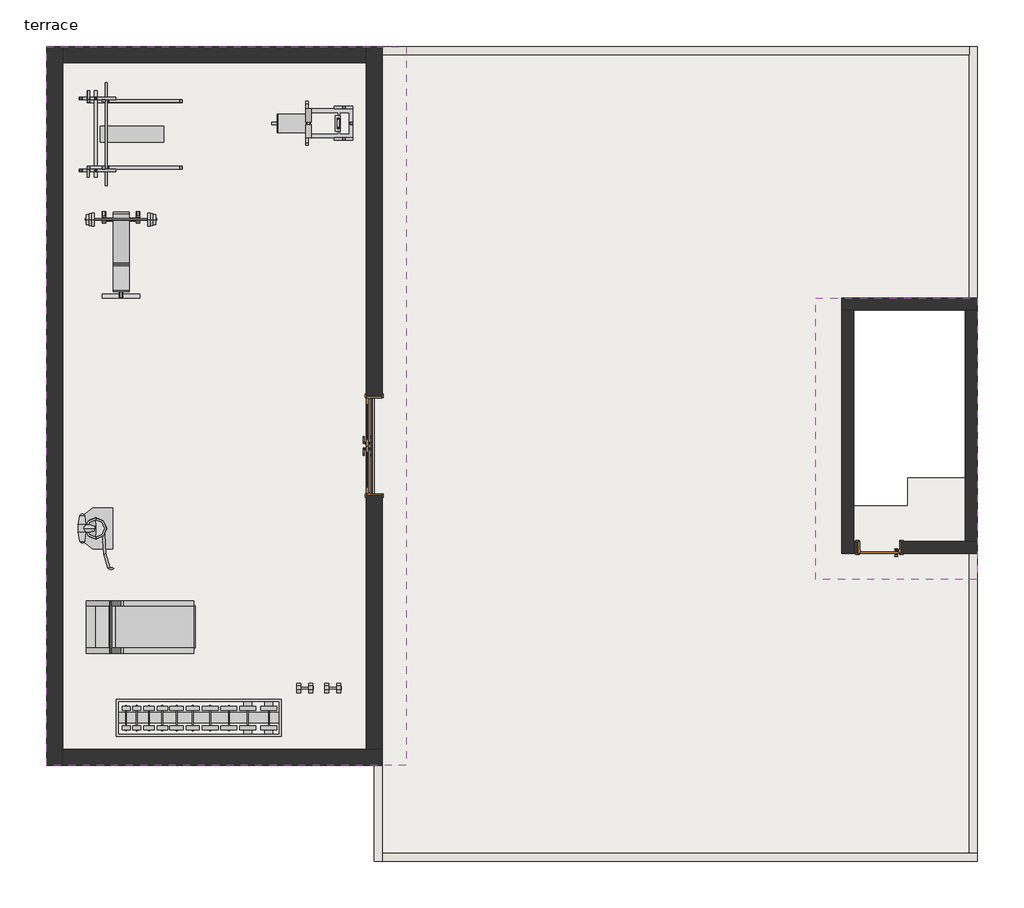
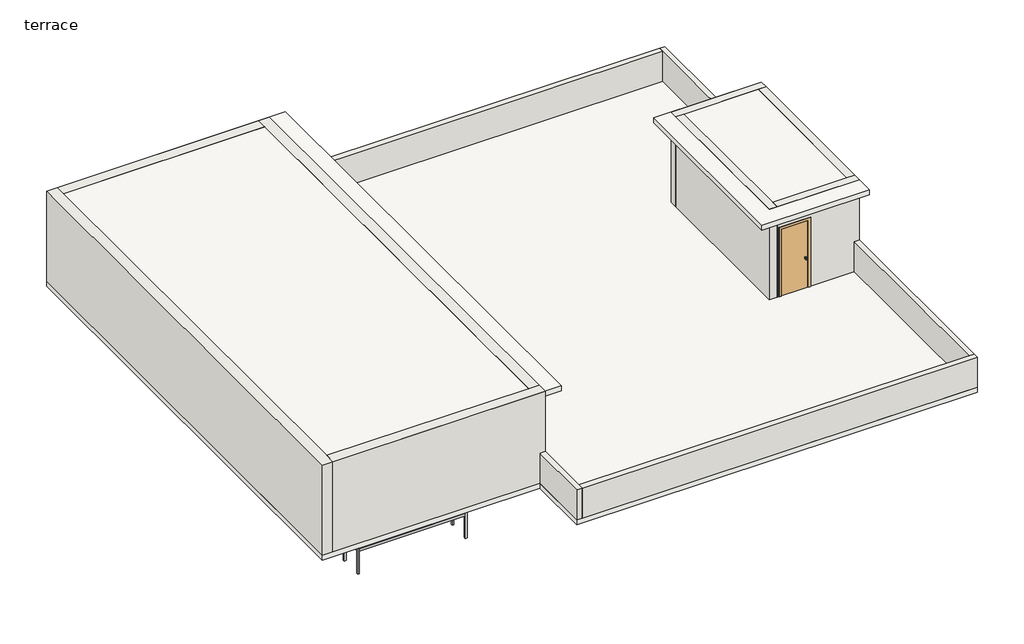
# One storey, incomplete: 13 walls, 7 proxies, 3 slabs, 2 doors, 1 furniture element.
"""IFC4 building model written with IfcOpenShell, lengths in millimetres."""

from ifc_helpers import new_model, si_unit, frame, origin, place, context, project, spatial, polyline, outline, extrude, faceted_brep, transform, mapped, element, save
from components import generic_models_aa191242, specialty_equipment_60971a7b, generic_models_59bf1475, specialty_equipment_45cd0696, lifting_bench_lifting_bench_243d69f3, treadmill_metric_18420_treadmill_metric_18420_532483b1, door_c1904fbe, door_d1f25229, gym_weight_bench_set_14865_gym_weight_bench_set_14865_0f5544b4

model = new_model("IFC4")

# Units and contexts
model_context = context("Model", 3, world=origin())
ifc_project = project(units=[si_unit("LENGTHUNIT", "METRE", prefix="MILLI")], contexts=[model_context])

# Site, building, storey
site = spatial("IfcSite", under=ifc_project)
building = spatial("IfcBuilding", under=site)
storey = spatial("IfcBuildingStorey", under=building, Name="terrace", Elevation=10210.8)

# Proxies
placement = place(None, origin())
generic_models_shape = generic_models_aa191242(model_context)
element("IfcBuildingElementProxy", 1, Name="Generic Models", at=placement, inside=storey, context=model_context, shape_type="MappedRepresentation", body=[
    mapped(generic_models_shape, transform((-7089.7739162, -2120.8339187, 10210.8), x_axis=(0.0, 1.0, 0.0), y_axis=(-1.0, 0.0, 0.0), z_axis=(0.0, 0.0, 1.0))),
])
specialty_equipment_shape = specialty_equipment_60971a7b(model_context)
element("IfcBuildingElementProxy", 2, Name="Specialty Equipment", at=placement, inside=storey, context=model_context, shape_type="MappedRepresentation", body=[
    mapped(specialty_equipment_shape, transform((-5667.3739162, -5930.8339187, 10210.8), x_axis=(1.0, 0.0, 0.0), y_axis=(0.0, 1.0, 0.0), z_axis=(0.0, 0.0, 1.0))),
])
generic_models_2_shape = generic_models_59bf1475(model_context)
element("IfcBuildingElementProxy", 3, Name="Generic Models", at=placement, inside=storey, context=model_context, shape_type="MappedRepresentation", body=[
    mapped(generic_models_2_shape, transform((-2644.7739162, -5168.8339187, 10210.8), x_axis=(1.0, 0.0, 0.0), y_axis=(0.0, 1.0, 0.0), z_axis=(0.0, 0.0, 1.0))),
])
element("IfcBuildingElementProxy", 4, Name="Generic Models", at=placement, inside=storey, context=model_context, shape_type="MappedRepresentation", body=[
    mapped(generic_models_2_shape, transform((-3178.1739162, -5168.8339187, 10210.8), x_axis=(1.0, 0.0, 0.0), y_axis=(0.0, 1.0, 0.0), z_axis=(0.0, 0.0, 1.0))),
])
specialty_equipment_2_shape = specialty_equipment_45cd0696(model_context)
element("IfcBuildingElementProxy", 5, Name="Specialty Equipment", at=placement, inside=storey, context=model_context, shape_type="MappedRepresentation", body=[
    mapped(specialty_equipment_2_shape, transform((-2429.0078371, 5204.0745668, 10210.8), x_axis=(0.0, 1.0, 0.0), y_axis=(-1.0, 0.0, 0.0), z_axis=(0.0, 0.0, 1.0))),
])
lifting_bench_lifting_bench_shape = lifting_bench_lifting_bench_243d69f3(model_context)
element("IfcBuildingElementProxy", 6, Name="Lifting Bench : Lifting Bench", ObjectType="Lifting Bench : Lifting Bench", at=placement, inside=storey, context=model_context, shape_type="MappedRepresentation", body=[
    mapped(lifting_bench_lifting_bench_shape, transform((-6964.4872648, 2273.3660813, 10210.8), x_axis=(1.0, 0.0, 0.0), y_axis=(0.0, 1.0, 0.0), z_axis=(0.0, 0.0, 1.0))),
])
treadmill_metric_18420_treadmill_metric_18420_shape = treadmill_metric_18420_treadmill_metric_18420_532483b1(model_context)
element("IfcBuildingElementProxy", 7, Name="Treadmill_metric_18420 : Treadmill_metric_18420", ObjectType="Treadmill_metric_18420 : Treadmill_metric_18420", at=placement, inside=storey, context=model_context, shape_type="MappedRepresentation", body=[
    mapped(treadmill_metric_18420_treadmill_metric_18420_shape, transform((-7267.5739162, -3640.5277171, 10210.8), x_axis=(0.0, -1.0, 0.0), y_axis=(1.0, 0.0, 0.0), z_axis=(0.0, 0.0, 1.0))),
])

# Doors
door_shape = door_c1904fbe(model_context)
element("IfcDoor", 8, ObjectType="Door-Exterior-Double-Full Glass-Wood_Clad : 72\" x 84\"", at=placement, inside=storey, context=model_context, shape_type="MappedRepresentation", body=[
    mapped(door_shape, transform((-1784.3489162, -546.0339187, 10210.8), x_axis=(0.0, 1.0, 0.0), y_axis=(-1.0, 0.0, 0.0), z_axis=(0.0, 0.0, 1.0))),
])
door_2_shape = door_d1f25229(model_context)
element("IfcDoor", 9, ObjectType="Door-Interior-Single-Flush_Panel-Wood : 30\" x 80\"", at=placement, inside=storey, context=model_context, shape_type="MappedRepresentation", body=[
    mapped(door_2_shape, transform((7858.1260838, -2492.3089187, 10210.8), x_axis=(-1.0, 0.0, 0.0), y_axis=(0.0, -1.0, 0.0), z_axis=(0.0, 0.0, 1.0))),
])

# Furniture
gym_weight_bench_set_14865_gym_weight_bench_set_14865_shape = gym_weight_bench_set_14865_gym_weight_bench_set_14865_0f5544b4(model_context)
element("IfcFurniture", 10, ObjectType="Gym_weight_bench_set_14865 : Gym_weight_bench_set_14865", at=placement, inside=storey, context=model_context, shape_type="MappedRepresentation", body=[
    mapped(gym_weight_bench_set_14865_gym_weight_bench_set_14865_shape, transform((-5438.7739162, 4737.1660813, 10210.8), x_axis=(0.0, 1.0, 0.0), y_axis=(-1.0, 0.0, 0.0), z_axis=(0.0, 0.0, 1.0))),
])

# Slabs
element("IfcSlab", 11, ObjectType="Generic - 6\"", at=placement, inside=storey, context=model_context, shape_type="SweptSolid", body=[
    extrude(outline(polyline([(-8029.5739162, 7073.9660813), (9725.0260838, 7073.9660813), (9725.0260838, 2044.7660813), (7362.8260838, 2044.7660813), (7362.8260838, -1689.0339187), (8391.5260838, -1689.0339187), (8391.5260838, -1157.2214187), (9725.0260838, -1157.2214187), (9725.0260838, -8470.8339187), (-1781.1739162, -8470.8339187), (-1781.1739162, -6642.0339187), (-8029.5739162, -6642.0339187), (-8029.5739162, 7073.9660813)])), frame((0.0, 0.0, 10058.4), z_axis=(0.0, 0.0, 1.0), x_axis=(1.0, 0.0, 0.0)), (0.0, 0.0, 1.0), 152.4),
])
element("IfcSlab", 12, ObjectType="Generic - 6\"", at=placement, inside=storey, context=model_context, shape_type="SweptSolid", body=[
    extrude(outline(polyline([(9725.0260838, 2273.3660813), (9725.0260838, -3098.7339187), (6638.9260838, -3098.7339187), (6638.9260838, 2273.3660813), (9725.0260838, 2273.3660813)])), frame((0.0, 0.0, 12801.6), z_axis=(0.0, 0.0, 1.0), x_axis=(1.0, 0.0, 0.0)), (0.0, 0.0, 1.0), 152.4),
])
element("IfcSlab", 13, ObjectType="Generic - 6\"", at=placement, inside=storey, context=model_context, shape_type="SweptSolid", body=[
    extrude(outline(polyline([(-1171.5739162, 7073.9660813), (-1171.5739162, -6642.0339187), (-8029.5739162, -6642.0339187), (-8029.5739162, 7073.9660813), (-1171.5739162, 7073.9660813)])), frame((0.0, 0.0, 12801.6), z_axis=(0.0, 0.0, 1.0), x_axis=(1.0, 0.0, 0.0)), (0.0, 0.0, 1.0), 152.4),
])

# Walls
element("IfcWall", 14, ObjectType="Generic - 12\"", at=placement, inside=storey, context=model_context, shape_type="Brep", body=[
    faceted_brep([(-8029.5739162, 7073.8999498, 10210.8), (-8029.5739162, -6642.0339187, 10210.8), (-8029.5739162, -6642.0339187, 12954.0), (-8029.5739162, 7073.8999498, 12954.0), (-7724.7739162, 7073.8999498, 10210.8), (-7724.7739162, 7073.8999498, 12954.0), (-7724.7739162, 6769.0999498, 12954.0), (-7724.7739162, -6337.2339187, 12954.0), (-7724.7739162, -6642.0339187, 12954.0), (-7724.7739162, -6642.0339187, 10210.8), (-7724.7739162, -6337.2339187, 10210.8), (-7724.7739162, 6769.0999498, 10210.8)], [[[0, 1, 2, 3]], [[4, 5, 6, 7, 8, 9, 10, 11]], [[1, 0, 4, 11, 10, 9]], [[3, 2, 8, 7, 6, 5]], [[2, 1, 9, 8]], [[0, 3, 5, 4]]]),
])
element("IfcWall", 15, ObjectType="Generic - 12\"", at=placement, inside=storey, context=model_context, shape_type="Brep", body=[
    faceted_brep([(-7724.7739162, -6642.0339187, 10210.8), (-1781.1739162, -6642.0339187, 10210.8), (-1781.1739162, -6642.0339187, 11125.2), (-1628.7739162, -6642.0339187, 11125.2), (-1628.7739162, -6642.0339187, 12954.0), (-7724.7739162, -6642.0339187, 12954.0), (-7724.7739162, -6337.2339187, 10210.8), (-7724.7739162, -6337.2339187, 12954.0), (-1933.5739162, -6337.2339187, 12954.0), (-1628.7739162, -6337.2339187, 12954.0), (-1628.7739162, -6337.2339187, 11125.2), (-1781.1739162, -6337.2339187, 11125.2), (-1781.1739162, -6337.2339187, 10210.8), (-1933.5739162, -6337.2339187, 10210.8)], [[[0, 1, 2, 3, 4, 5]], [[6, 7, 8, 9, 10, 11, 12, 13]], [[1, 0, 6, 13, 12]], [[5, 4, 9, 8, 7]], [[0, 5, 7, 6]], [[10, 3, 2, 11]], [[2, 1, 12, 11]], [[4, 3, 10, 9]]]),
])
element("IfcWall", 16, ObjectType="Generic - 12\"", at=placement, inside=storey, context=model_context, shape_type="SweptSolid", body=[
    extrude(outline(polyline([(-1933.5739162, 6769.0999498), (-7724.7739162, 6769.0999498), (-7724.7739162, 7073.8999498), (-1933.5739162, 7073.8999498), (-1933.5739162, 6769.0999498)])), frame((0.0, 0.0, 10210.8), z_axis=(0.0, 0.0, 1.0), x_axis=(1.0, 0.0, 0.0)), (0.0, 0.0, 1.0), 2743.2),
])
element("IfcWall", 17, ObjectType="Generic - 12\"", at=placement, inside=storey, context=model_context, shape_type="Brep", body=[
    faceted_brep([(-1933.5739162, -6337.2339187, 12954.0), (-1933.5739162, 6769.0999498, 12954.0), (-1933.5739162, 7073.9660813, 12954.0), (-1933.5739162, 7073.9660813, 10210.8), (-1933.5739162, 6769.0999498, 10210.8), (-1933.5739162, 393.7660813, 10210.8), (-1933.5739162, 393.7660813, 12369.8), (-1933.5739162, -1485.8339187, 12369.8), (-1933.5739162, -1485.8339187, 10210.8), (-1933.5739162, -6337.2339187, 10210.8), (-1628.7739162, 7073.9660813, 12954.0), (-1628.7739162, -6337.2339187, 12954.0), (-1628.7739162, -6337.2339187, 11125.2), (-1628.7739162, -6337.2339187, 10210.8), (-1628.7739162, -1485.8339187, 10210.8), (-1628.7739162, -1485.8339187, 12369.8), (-1628.7739162, 393.7660813, 12369.8), (-1628.7739162, 393.7660813, 10210.8), (-1628.7739162, 6921.5660813, 10210.8), (-1628.7739162, 7073.9660813, 10210.8), (-1628.7739162, 7073.9660813, 11125.2), (-1781.1739162, -6337.2339187, 10210.8)], [[[0, 1, 2, 3, 4, 5, 6, 7, 8, 9]], [[10, 11, 12, 13, 14, 15, 16, 17, 18, 19, 20]], [[3, 19, 18, 17, 5, 4]], [[13, 21, 9, 8, 14]], [[2, 1, 0, 11, 10]], [[3, 2, 10, 20, 19]], [[0, 9, 21, 13, 12, 11]], [[16, 6, 5, 17]], [[6, 16, 15, 7]], [[7, 15, 14, 8]]]),
])
element("IfcWall", 18, ObjectType="Generic - 6\"", at=placement, inside=storey, context=model_context, shape_type="Brep", body=[
    faceted_brep([(9725.0260838, 2273.3660813, 10210.8), (9725.0260838, 7073.9660813, 10210.8), (9725.0260838, 7073.9660813, 11125.2), (9725.0260838, 2273.3660813, 11125.2), (9572.6260838, 2273.3660813, 10210.8), (9572.6260838, 2273.3660813, 11125.2), (9572.6260838, 6921.5660813, 11125.2), (9572.6260838, 7073.9660813, 11125.2), (9572.6260838, 7073.9660813, 10210.8), (9572.6260838, 6921.5660813, 10210.8)], [[[0, 1, 2, 3]], [[4, 5, 6, 7, 8, 9]], [[1, 0, 4, 9, 8]], [[3, 2, 7, 6, 5]], [[0, 3, 5, 4]], [[2, 1, 8, 7]]]),
])
element("IfcWall", 19, ObjectType="Generic - 6\"", at=placement, inside=storey, context=model_context, shape_type="SweptSolid", body=[
    extrude(outline(polyline([(-1628.7739162, 7073.9660813), (9572.6260838, 7073.9660813), (9572.6260838, 6921.5660813), (-1628.7739162, 6921.5660813), (-1628.7739162, 7073.9660813)])), frame((0.0, 0.0, 10210.8), z_axis=(0.0, 0.0, 1.0), x_axis=(1.0, 0.0, 0.0)), (0.0, 0.0, 1.0), 914.4),
])
element("IfcWall", 20, ObjectType="Generic - 6\"", at=placement, inside=storey, context=model_context, shape_type="Brep", body=[
    faceted_brep([(-1781.1739162, -6337.2339187, 10210.8), (-1781.1739162, -6642.0339187, 10210.8), (-1781.1739162, -8470.8339187, 10210.8), (-1781.1739162, -8470.8339187, 11125.2), (-1781.1739162, -6642.0339187, 11125.2), (-1781.1739162, -6337.2339187, 11125.2), (-1628.7739162, -6337.2339187, 10210.8), (-1628.7739162, -6337.2339187, 11125.2), (-1628.7739162, -6642.0339187, 11125.2), (-1628.7739162, -8318.4339187, 11125.2), (-1628.7739162, -8470.8339187, 11125.2), (-1628.7739162, -8470.8339187, 10210.8), (-1628.7739162, -8318.4339187, 10210.8)], [[[0, 1, 2, 3, 4, 5]], [[6, 7, 8, 9, 10, 11, 12]], [[2, 1, 0, 6, 12, 11]], [[5, 4, 3, 10, 9, 8, 7]], [[3, 2, 11, 10]], [[0, 5, 7, 6]]]),
])
element("IfcWall", 21, ObjectType="Generic - 6\"", at=placement, inside=storey, context=model_context, shape_type="Brep", body=[
    faceted_brep([(-1628.7739162, -8470.8339187, 10210.8), (9725.0260838, -8470.8339187, 10210.8), (9725.0260838, -8470.8339187, 11125.2), (-1628.7739162, -8470.8339187, 11125.2), (-1628.7739162, -8318.4339187, 10210.8), (-1628.7739162, -8318.4339187, 11125.2), (9572.6260838, -8318.4339187, 11125.2), (9725.0260838, -8318.4339187, 11125.2), (9725.0260838, -8318.4339187, 10210.8), (9572.6260838, -8318.4339187, 10210.8)], [[[0, 1, 2, 3]], [[4, 5, 6, 7, 8, 9]], [[1, 0, 4, 9, 8]], [[3, 2, 7, 6, 5]], [[0, 3, 5, 4]], [[2, 1, 8, 7]]]),
])
element("IfcWall", 22, ObjectType="Generic - 6\"", at=placement, inside=storey, context=model_context, shape_type="SweptSolid", body=[
    extrude(outline(polyline([(9725.0260838, -2603.4339187), (9725.0260838, -8318.4339187), (9572.6260838, -8318.4339187), (9572.6260838, -2603.4339187), (9725.0260838, -2603.4339187)])), frame((0.0, 0.0, 10210.8), z_axis=(0.0, 0.0, 1.0), x_axis=(1.0, 0.0, 0.0)), (0.0, 0.0, 1.0), 914.4),
])
element("IfcWall", 23, ObjectType="Generic - 9\"", at=placement, inside=storey, context=model_context, shape_type="Brep", body=[
    faceted_brep([(9725.0260838, 2273.3660813, 12954.0), (9725.0260838, 2273.3660813, 11125.2), (9725.0260838, 2273.3660813, 10210.8), (9572.6260838, 2273.3660813, 10210.8), (7134.2260838, 2273.3660813, 10210.8), (7134.2260838, 2273.3660813, 12954.0), (9725.0260838, 2044.7660813, 10210.8), (9725.0260838, 2044.7660813, 12954.0), (9496.4260838, 2044.7660813, 12954.0), (7362.8260838, 2044.7660813, 12954.0), (7134.2260838, 2044.7660813, 12954.0), (7134.2260838, 2044.7660813, 10210.8), (7362.8260838, 2044.7660813, 10210.8), (9496.4260838, 2044.7660813, 10210.8)], [[[0, 1, 2, 3, 4, 5]], [[6, 7, 8, 9, 10, 11, 12, 13]], [[4, 3, 2, 6, 13, 12, 11]], [[0, 5, 10, 9, 8, 7]], [[5, 4, 11, 10]], [[0, 7, 6, 2, 1]]]),
])
element("IfcWall", 24, ObjectType="Generic - 9\"", at=placement, inside=storey, context=model_context, shape_type="Brep", body=[
    faceted_brep([(7134.2260838, 2044.7660813, 10210.8), (7134.2260838, -2603.4339187, 10210.8), (7134.2260838, -2603.4339187, 12954.0), (7134.2260838, 2044.7660813, 12954.0), (7362.8260838, 2044.7660813, 10210.8), (7362.8260838, 2044.7660813, 12954.0), (7362.8260838, -2374.8339187, 12954.0), (7362.8260838, -2603.4339187, 12954.0), (7362.8260838, -2603.4339187, 10210.8), (7362.8260838, -2374.8339187, 10210.8)], [[[0, 1, 2, 3]], [[4, 5, 6, 7, 8, 9]], [[1, 0, 4, 9, 8]], [[3, 2, 7, 6, 5]], [[0, 3, 5, 4]], [[2, 1, 8, 7]]]),
])
element("IfcWall", 25, ObjectType="Generic - 9\"", at=placement, inside=storey, context=model_context, shape_type="Brep", body=[
    faceted_brep([(9725.0260838, -2603.4339187, 12954.0), (7362.8260838, -2603.4339187, 12954.0), (7362.8260838, -2603.4339187, 10210.8), (7451.7260838, -2603.4339187, 10210.8), (7451.7260838, -2603.4339187, 12268.2), (8264.5260838, -2603.4339187, 12268.2), (8264.5260838, -2603.4339187, 10210.8), (9572.6260838, -2603.4339187, 10210.8), (9725.0260838, -2603.4339187, 10210.8), (9725.0260838, -2603.4339187, 11125.2), (7362.8260838, -2374.8339187, 12954.0), (9496.4260838, -2374.8339187, 12954.0), (9725.0260838, -2374.8339187, 12954.0), (9725.0260838, -2374.8339187, 10210.8), (9496.4260838, -2374.8339187, 10210.8), (8264.5260838, -2374.8339187, 10210.8), (8264.5260838, -2374.8339187, 12268.2), (7451.7260838, -2374.8339187, 12268.2), (7451.7260838, -2374.8339187, 10210.8), (7362.8260838, -2374.8339187, 10210.8)], [[[0, 1, 2, 3, 4, 5, 6, 7, 8, 9]], [[10, 11, 12, 13, 14, 15, 16, 17, 18, 19]], [[2, 19, 18, 3]], [[13, 8, 7, 6, 15, 14]], [[1, 0, 12, 11, 10]], [[2, 1, 10, 19]], [[8, 13, 12, 0, 9]], [[17, 4, 3, 18]], [[4, 17, 16, 5]], [[5, 16, 15, 6]]]),
])
element("IfcWall", 26, ObjectType="Generic - 9\"", at=placement, inside=storey, context=model_context, shape_type="SweptSolid", body=[
    extrude(outline(polyline([(9725.0260838, 2044.7660813), (9725.0260838, -2374.8339187), (9496.4260838, -2374.8339187), (9496.4260838, 2044.7660813), (9725.0260838, 2044.7660813)])), frame((0.0, 0.0, 10210.8), z_axis=(0.0, 0.0, 1.0), x_axis=(1.0, 0.0, 0.0)), (0.0, 0.0, 1.0), 2743.2),
])

save(model, "model.ifc")

# Revit data of these elements
# Type
#   Rope Hide [instance] = yes
#   Rope [instance] = Rope
#   Bollard = Bollard
#   Default Elevation = 0
# Type
#   Default Elevation = 0
# Type
#   Text Depth = 0' - 0 1/8"
#   Text Color = none
#   Dumbell Material = none
#   Default Elevation = 0
# Type
#   Assembly Code = "E1090"
#   Top width = 1' - 0.07125"
#   Height = 10' - 9.92126"
#   Frame thickness = 0' - 1.9685"
#   vinyl = Plastic - Black
#   Metal Material = Metal - painted
#   Metal - painted = Metal - painted
#   Black = none
#   Default Elevation = 0
# Type "Lifting Bench : Lifting Bench"
#   Assembly Code = "E1090"
#   Default Elevation = 0
# Type "Treadmill_metric_18420 : Treadmill_metric_18420"
#   Assembly Code = "E1090"
#   width = 3' - 3.37008"
#   belt width = 2' - 7.49606"
#   Lenght = 6' - 8.70866"
#   Default Elevation = 0
# Type "Door-Exterior-Double-Full Glass-Wood_Clad : 72\" x 84\""
#   Type Mark = "13"
#   Assembly Code = "B2030100"
#   Analytic Construction = "French door, wood frame with double glass"
#   Top Rail = 0' - 4 11/16"
#   Threshold Offset [instance default] = 0' - 0 1/2"
#   Thickness = 0' - 1 3/8"
#   Thermal Resistance (R) = 1.9158 (h·ft²·°F)/BTU
#   Swing Angle [instance default] = 90.00°
#   Stiles = 0' - 4 3/4"
#   Rough Width = 6' - 2"
#   Rough Height = 7' - 1"
#   Panel Width = 3' - 0"
#   Door Offset [instance default] = 0' - 0"
#   Height = 7' - 0"
#   Width = 6' - 0"
#   Heat Transfer Coefficient (U) = 0.5220 BTU/(h·ft²·°F)
#   Bottom Rail = 0' - 9 1/8"
#   Exterior Trim [instance default] = yes
#   Threshold [instance default] = yes
#   Show Grill [instance default] = yes
#   Function = 1
#   Trim Material = Cherry
#   Threshold Material = Cherry
#   Panel Material = Cherry
#   Glazing = Glass
#   Frame Material = Cherry
#   Door Handle Material = Aluminum
#   Visual Light Transmittance = 0
#   Solar Heat Gain Coefficient = 0
#   Wall Closure = (empty or 0)
#   Construction Type = (empty or 0)
# Type "Door-Interior-Single-Flush_Panel-Wood : 30\" x 80\""
#   Type Mark = "12"
#   Assembly Code = "C1020300"
#   Analytic Construction = "Wooden"
#   Thickness = 0' - 1 3/8"
#   Thermal Resistance (R) = 2.5876 (h·ft²·°F)/BTU
#   Swing Angle [instance default] = 90.00°
#   Rough Width = 2' - 8"
#   Rough Height = 6' - 9"
#   Height = 6' - 8"
#   Width = 2' - 6"
#   Heat Transfer Coefficient (U) = 0.3865 BTU/(h·ft²·°F)
#   Trim Material = Cherry
#   Panel Material = Cherry
#   Frame Material = Cherry
#   Door Handle Material = Aluminum
#   Visual Light Transmittance = 0
#   Solar Heat Gain Coefficient = 0
#   Wall Closure = (empty or 0)
#   Function = (empty or 0)
# Type "Gym_weight_bench_set_14865 : Gym_weight_bench_set_14865"
#   Default Elevation = 0
# Type "Generic - 6\""
#   Assembly Code = "B1010"
#   Function = 0
#   Layers, outside or top first: 0' - 6" no material (function 1)
# Type "Generic - 12\""
#   Assembly Code = "B2010"
#   Layers, outside or top first: 1' - 0" no material (function 1)
# Type "Generic - 6\""
#   Assembly Code = "B2010"
#   Layers, outside or top first: 0' - 6" no material (function 1)
# Type "Generic - 9\""
#   Assembly Code = "B2010"
#   Layers, outside or top first: 0' - 9" no material (function 1)
# Element 1 (IfcBuildingElementProxy)
#   Rope Hide = yes
#   Rope = Rope
#   Phase Created = New Construction
#   Materials on its faces: "Bollard", "Rope"
# Elements 2, 3, 4 (IfcBuildingElementProxy)
#   Phase Created = New Construction
# Element 5 (IfcBuildingElementProxy)
#   Phase Created = New Construction
#   Materials on its faces: "Metal - painted", "Plastic - Black"
# Element 6 (IfcBuildingElementProxy, "Lifting Bench : Lifting Bench")
#   Phase Created = New Construction
#   Materials on its faces: "Plastic - Black"
# Element 7 (IfcBuildingElementProxy, "Treadmill_metric_18420 : Treadmill_metric_18420")
#   Phase Created = New Construction
#   Materials on its faces: "Metal - Steel", "Default"
# Element 8 (IfcDoor, "Door-Exterior-Double-Full Glass-Wood_Clad : 72\" x 84\"")
#   Threshold Offset = 0' - 0 1/2"
#   Swing Angle = 90.00°
#   Door Offset = 0' - 0"
#   Threshold = yes
#   Show Grill = yes
#   Exterior Trim = yes
#   Phase Created = New Construction
#   Materials on its faces: "Cherry", "Aluminum", "Glass"
# Element 9 (IfcDoor, "Door-Interior-Single-Flush_Panel-Wood : 30\" x 80\"")
#   Swing Angle = 90.00°
#   Phase Created = New Construction
#   Materials on its faces: "Cherry", "Aluminum"
# Element 10 (IfcFurniture, "Gym_weight_bench_set_14865 : Gym_weight_bench_set_14865")
#   Phase Created = New Construction
#   Materials on its faces: "black", "silver", "white"
# Element 11 (IfcSlab, "Generic - 6\"")
#   built-in parameter 1001955 = 1.5708 (stored number, unit not read)
#   Height Offset From Level = 0' - 0"
#   Phase Created = New Construction
#   Materials on its faces: "Default Floor"
# Elements 12, 13 (IfcSlab, "Generic - 6\"")
#   Height Offset From Level = 9' - 0"
#   Phase Created = New Construction
#   Materials on its faces: "Default Floor"
# Elements 14, 15, 16, 17 (IfcWall, "Generic - 12\"")
#   Top Offset = 0' - 0"
#   Base Offset = 0' - 0"
#   wall height = 9' - 0"
#   Phase Created = New Construction
#   Base Constraint = terrace
#   Top Constraint = stair head roof
#   Materials on its faces: "Default Wall"
# Elements 18, 19, 20, 21, 22 (IfcWall, "Generic - 6\"")
#   Top Offset = 0' - 0"
#   Base Offset = 0' - 0"
#   wall height = 3' - 0"
#   Phase Created = New Construction
#   Base Constraint = terrace
#   Materials on its faces: "Default Wall"
# Elements 23, 24, 25, 26 (IfcWall, "Generic - 9\"")
#   Top Offset = 0' - 0"
#   Base Offset = 0' - 0"
#   wall height = 9' - 0"
#   Phase Created = New Construction
#   Base Constraint = terrace
#   Top Constraint = stair head roof
#   Materials on its faces: "Default Wall"
# Materials
#   "Rope": class "Generic", colour RGB 192 128 68, transparency 0, Cost = 0
#   "Bollard": class "Generic", colour RGB 226 219 42, transparency 0, Cost = 0
#   "Plastic - Black": colour RGB 0 0 0, transparency 0
#   "Metal - painted": colour RGB 247 247 239, transparency 0
#   "Cherry": class "Wood", colour RGB 226 177 128, transparency 0, Description = "Prunus Serotina", Cost = 0
#   "Glass": class "Glass", colour RGB 0 128 192, transparency 0.75, Description = "Soda Lime Glass", Cost = 0
#   "Aluminum": class "Metal", colour RGB 247 247 247, transparency 0, Description = "Aluminum 6061", Cost = 0
#   "Metal - Steel": colour RGB 247 247 247, transparency 0
#   "Default": colour RGB 127 127 127, transparency 0, Cost = 0
#   "black": class "Metal", colour RGB 0 0 0, transparency 0
#   "silver": class "Generic", colour RGB 120 120 120, transparency 0, Cost = 0
#   "white": class "Generic", colour RGB 120 120 120, transparency 0, Cost = 0
#   "Default Floor": colour RGB 128 128 128, transparency 0, Cost = 0
#   "Default Wall": colour RGB 128 128 128, transparency 0, Cost = 0
